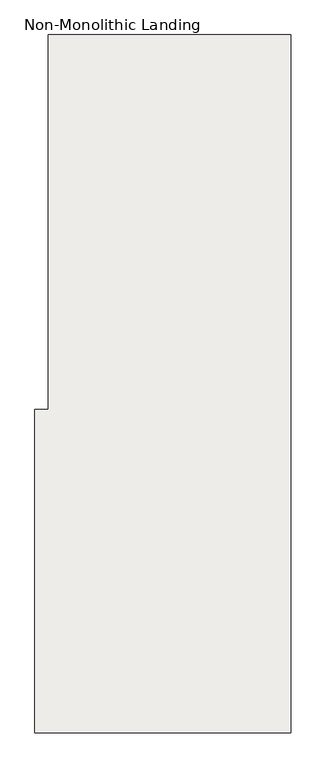
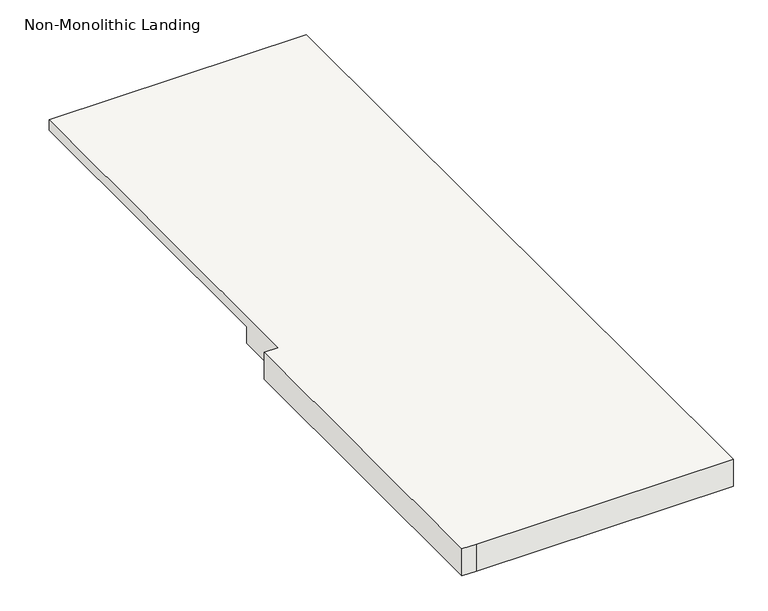
"""IFC4 building model written with IfcOpenShell, lengths in millimetres: slab geometry, Non-Monolithic Landing."""

from ifc_helpers import new_model, si_unit, origin, place, context, project, spatial, faceted_brep, source, transform, mapped, element, save


def non_monolithic_landing_a944a33a(model_context):
    return source(origin(), model_context, "Body", "Brep", [
        faceted_brep([(-3732.7409298, -3238.4779636, 1581.15), (-3707.3409298, -3238.4779636, 1555.75), (-3707.3409298, -3848.0779636, 1555.75), (-3732.7409298, -3848.0779636, 1581.15), (-3732.7409298, -3945.3664375, 1600.2), (-3758.1409298, -3945.3664375, 1600.2), (-3758.1409298, -4554.9664375, 1600.2), (-3732.7409298, -4554.9664375, 1600.2), (-3275.5409298, -4554.9664375, 1600.2), (-3275.5409298, -3238.4779636, 1600.2), (-3732.7409298, -3238.4779636, 1600.2), (-3707.3409298, -3848.0779636, 1549.4), (-3707.3409298, -3238.4779636, 1549.4), (-3275.5409298, -3238.4779636, 1549.4), (-3275.5409298, -4554.9664375, 1549.4), (-3732.7409298, -4554.9664375, 1549.4), (-3758.1409298, -4554.9664375, 1549.4), (-3758.1409298, -3945.3664375, 1549.4), (-3732.7409298, -3945.3664375, 1549.4), (-3732.7409298, -3848.0779636, 1549.4)], [[[0, 1, 2, 3]], [[4, 5, 6, 7, 8, 9, 10]], [[11, 12, 13, 14, 15, 16, 17, 18, 19]], [[12, 11, 2, 1]], [[11, 19, 3, 2]], [[4, 10, 0, 3, 19, 18]], [[5, 4, 18, 17]], [[6, 5, 17, 16]], [[7, 6, 16, 15]], [[8, 7, 15, 14]], [[9, 8, 14, 13]], [[10, 9, 13, 12, 1, 0]]]),
    ])


if __name__ == "__main__":
    model = new_model("IFC4")
    model_context = context("Model", 3, world=origin())
    ifc_project = project(units=[si_unit("LENGTHUNIT", "METRE", prefix="MILLI")], contexts=[model_context])
    site = spatial("IfcSite", under=ifc_project)
    building = spatial("IfcBuilding", under=site)
    placement = place(None, origin())
    non_monolithic_landing_shape = non_monolithic_landing_a944a33a(model_context)
    element("IfcSlab", 1, ObjectType="Non-Monolithic Landing", at=placement, inside=building, context=model_context, shape_type="MappedRepresentation", body=[
        mapped(non_monolithic_landing_shape, transform((0.0, 0.0, 0.0), x_axis=(1.0, 0.0, 0.0), y_axis=(0.0, 1.0, 0.0), z_axis=(0.0, 0.0, 1.0))),
    ])
    save(model, "model.ifc")
